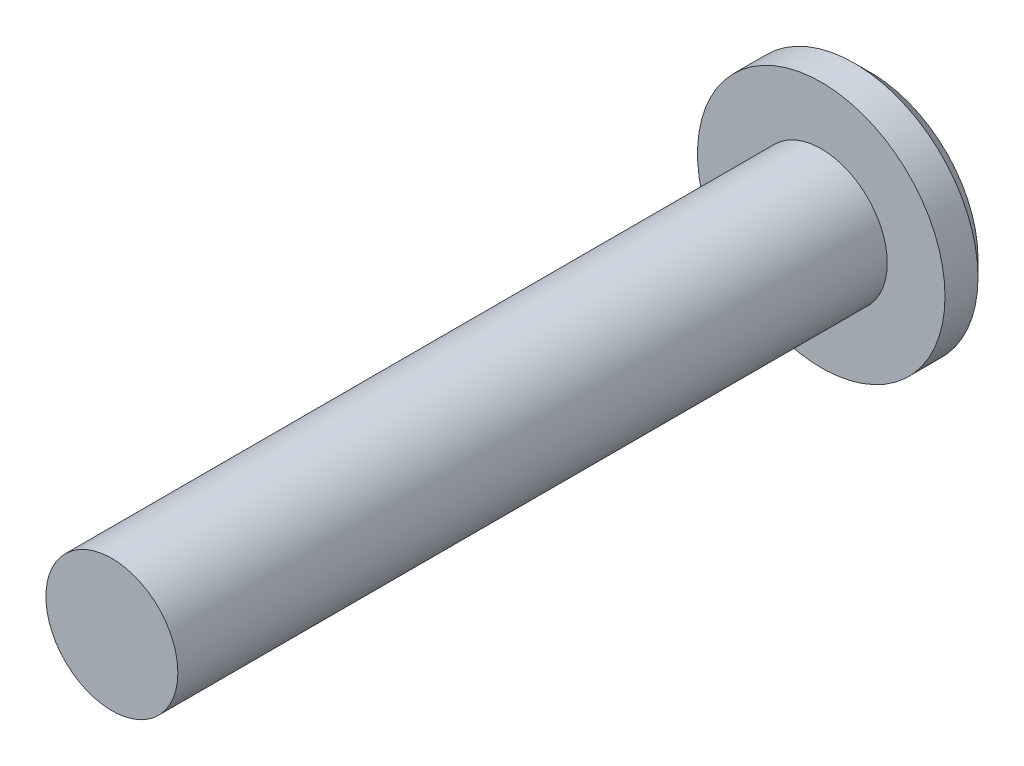
SolidWorks part; units mm, degrees
material "Plain Carbon Steel"
ref_plane "Front Plane" through (0, 0, 0) normal (0, 0, 1) x (1, 0, 0)
ref_plane "Top Plane" through (0, 0, 0) normal (0, 1, 0) x (1, 0, 0)
ref_plane "Right Plane" through (0, 0, 0) normal (1, 0, 0) x (0, 0, -1)
sketch "Head Profile Ø15" plane through (0, 0, 0) normal (0, 0, 1) x (1, 0, 0)
  circle A0 centre (0, 0) radius 7.5
  dimension "D1" = 15
extrude "Head Ø15x3" add sketch "Head Profile Ø15" along normal blind 3
sketch "Shank Profile Ø8" plane through (0, 0, 3) normal (0, 0, 1) x (1, 0, 0)
  circle A0 centre (0, 0) radius 4
  dimension "D1" = 8
extrude "Shank Ø8x43" add sketch "Shank Profile Ø8" along normal blind 43
cosmetic thread "Cosmetic Thread1"
chamfer "Head Chamfer 1x45°" distance 1 angle 45 1 edges at (7.5, 0, 0)
